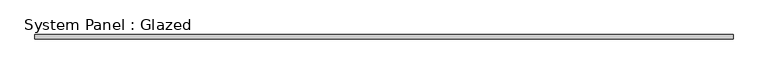
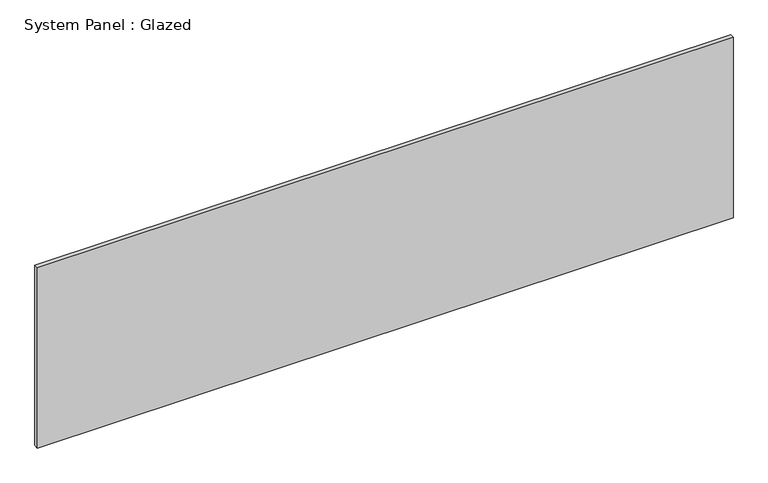
"""IFC4 building model written with IfcOpenShell, lengths in millimetres: plate geometry, System Panel : Glazed."""

from ifc_helpers import new_model, si_unit, origin, origin_with_axes, place, context, project, spatial, polyline, outline, extrude, source, transform, mapped, element, save


def system_panel_glazed_8d4a2524(model_context):
    return source(origin(), model_context, "Body", "SweptSolid", [
        extrude(outline(polyline([(1993.9, 19.05), (-1993.9, 19.05), (-1993.9, 44.45), (1993.9, 44.45), (1993.9, 19.05)])), origin_with_axes(), (0.0, 0.0, 1.0), 1092.2),
    ])


if __name__ == "__main__":
    model = new_model("IFC4")
    model_context = context("Model", 3, world=origin())
    ifc_project = project(units=[si_unit("LENGTHUNIT", "METRE", prefix="MILLI")], contexts=[model_context])
    site = spatial("IfcSite", under=ifc_project)
    building = spatial("IfcBuilding", under=site)
    placement = place(None, origin())
    system_panel_glazed_shape = system_panel_glazed_8d4a2524(model_context)
    element("IfcPlate", 1, ObjectType="System Panel : Glazed", at=placement, inside=building, context=model_context, shape_type="MappedRepresentation", body=[
        mapped(system_panel_glazed_shape, transform((0.0, 0.0, 0.0), x_axis=(1.0, 0.0, 0.0), y_axis=(0.0, 1.0, 0.0), z_axis=(0.0, 0.0, 1.0))),
    ])
    save(model, "model.ifc")

# Revit data of these elements
# Type "System Panel : Glazed"
#   Construction Type Id = "GSP4R"
#   Analytic Construction = "1/8 in Pilkington single glazing"
#   Visual Light Transmittance = 0.9
#   Solar Heat Gain Coefficient = 0.86
#   Heat Transfer Coefficient (U) = 1.18115 BTU/(h·ft²·°F)
# Element 1 (IfcPlate, "System Panel : Glazed")
#   Materials on its faces: "Glass"
# Materials
#   "Glass": class "Glass", colour RGB 0 128 192, transparency 0.75, Description = "Soda Lime Glass", Cost = 0
